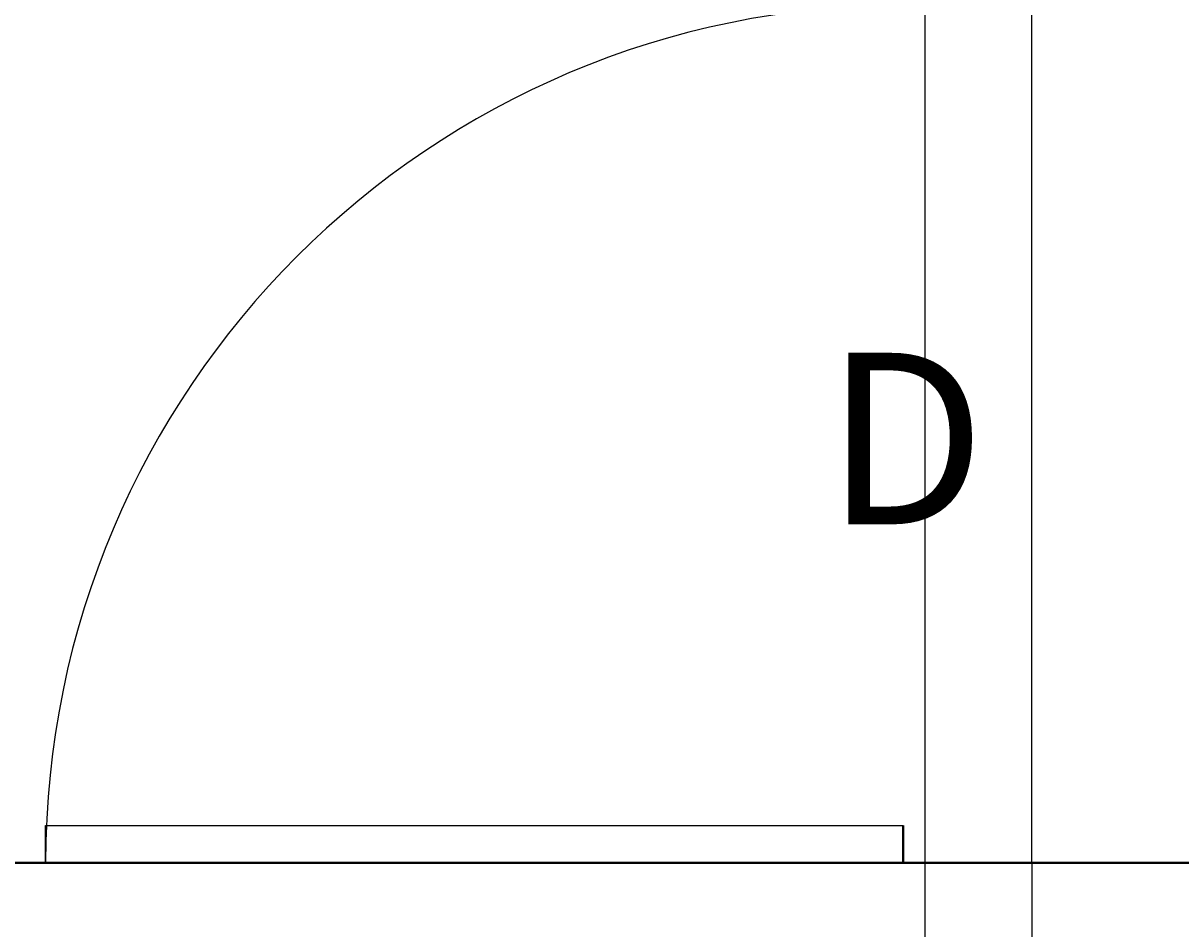
# Model space of a CAD drawing. Units: inches. Extents: x -301 to 715, y -607 to 364.
# Tile 65 of 141: x -93 to -39, y -218 to -176. Entities that reach past the tile are written whole.
import ezdxf

# ---------------------------------------------------------------- set-up
doc = ezdxf.new("R2010")
doc.units = ezdxf.units.IN
doc.header["$MEASUREMENT"] = 0
for name, color, linetype, lineweight in [('A-ANNO-DIMS', 2, 'Continuous', 18), ('A-ANNO-TEXT', 4, 'Continuous', 18), ('A-DOOR', 4, 'Continuous', 25), ('A-FLOR-STRS', 2, 'Continuous', 25), ('A-WALL', 3, 'Continuous', 40)]:
    doc.layers.add(name, color=color, linetype=linetype, lineweight=lineweight)
doc.styles.get("Standard").update_dxf_attribs({"font": 'arial.ttf'})
doc.dimstyles.get("Standard").update_dxf_attribs({"dimtxt": 0.18, "dimasz": 0.18, "dimexe": 0.18, "dimexo": 0.0625, "dimgap": 0.09, "dimtad": 0, "dimtih": 1, "dimtoh": 1, "dimdec": 1, "dimzin": 0, "dimdsep": 46, "dimlunit": 4, "dimtxsty": 'Standard', "dimcen": 0.09, "dimclrd": 3, "dimclre": 4, "dimclrt": 6, "dimadec": 0, "dimazin": 0, "dimtfac": 1, "dimtdec": 1, "dimtofl": 0, "dimtmove": 0, "dimatfit": 3, "dimfxl": 1, "dimtfill": 2, "dimtfillclr": 51, "dimtolj": 1, "dimtzin": 0, "dimarcsym": 0})

# ---------------------------------------------------------------- blocks, each defined once
blk = doc.blocks.new('*U4')
for p, q in [((0, 0), (0, -6)), ((40, 0), (40, -6))]:
    blk.add_line(p, q)
blk.add_lwpolyline([(0, 0), (0, 40), (1.75, 40), (1.75, 0)], close=True)
blk.add_arc((0, 0), 40, 0, 90)
blk = doc.blocks.new('ENTRY-STEPS-48')
for p, q in [((0, 27), (0, 18)), ((48, 27), (48, 18)), ((0, 18), (0, 9)), ((48, 9), (48, 18)), ((0, 9), (48, 9)), ((0, 9), (0, 0)), ((48, 0), (48, 9)), ((0, 0), (48, 0))]:
    blk.add_line(p, q)
blk = doc.blocks.new('*D151')
at = {"layer": 'A-ANNO-DIMS', "color": 4, "lineweight": -2, "transparency": 16777216}
for p, q in [((-204.603, -223.755), (-204.603, 359.612)), ((-45.603, -214.755), (-45.603, 359.612))]:
    blk.add_line(p, q, dxfattribs=at)
at = {"layer": 'A-ANNO-DIMS', "color": 3, "lineweight": -2, "transparency": 16777216}
for p, q in [((-204.423, 359.432), (-125.494, 359.432)), ((-45.783, 359.432), (-124.713, 359.432))]:
    blk.add_line(p, q, dxfattribs=at)
at = {"layer": 'A-ANNO-DIMS', "color": 3, "transparency": 16777216}
for points in [[(-204.423, 359.462), (-204.423, 359.402), (-204.603, 359.432)], [(-45.783, 359.462), (-45.783, 359.402), (-45.603, 359.432)]]:
    blk.add_solid(points, dxfattribs=at)
at = {"layer": 'Defpoints', "color": 0, "transparency": 16777216}
for p in [(-45.603, 359.432), (-45.603, -214.818), (-204.603, -223.818)]:
    blk.add_point(p, dxfattribs=at)
at = {"layer": 'A-ANNO-DIMS', "color": 6, "transparency": 16777216, "insert": (-125.103, 359.432), "char_height": 0.18, "attachment_point": 5, "bg_fill": 1, "box_fill_scale": 1.25, "bg_fill_color": 51, "bg_fill_transparency": 0}
blk.add_mtext('\\A1;13\'-3"', dxfattribs=at)
blk = doc.blocks.new('*D158')
at = {"layer": 'A-ANNO-DIMS', "color": 4, "lineweight": -2, "transparency": 16777216}
for p, q in [((-122.603, 221.62), (-122.603, -296.865)), ((-50.603, 221.62), (-50.603, -296.865))]:
    blk.add_line(p, q, dxfattribs=at)
at = {"layer": 'A-ANNO-DIMS', "color": 3, "lineweight": -2, "transparency": 16777216}
for p, q in [((-122.423, -296.685), (-86.933, -296.685)), ((-50.783, -296.685), (-86.274, -296.685))]:
    blk.add_line(p, q, dxfattribs=at)
at = {"layer": 'A-ANNO-DIMS', "color": 3, "transparency": 16777216}
for points in [[(-122.423, -296.655), (-122.423, -296.715), (-122.603, -296.685)], [(-50.783, -296.655), (-50.783, -296.715), (-50.603, -296.685)]]:
    blk.add_solid(points, dxfattribs=at)
at = {"layer": 'Defpoints', "color": 0, "transparency": 16777216}
for p in [(-122.603, 221.682), (-50.603, 221.682), (-50.603, -296.685)]:
    blk.add_point(p, dxfattribs=at)
at = {"layer": 'A-ANNO-DIMS', "color": 6, "transparency": 16777216, "insert": (-86.603, -296.685), "char_height": 0.18, "attachment_point": 5, "bg_fill": 1, "box_fill_scale": 1.25, "bg_fill_color": 51, "bg_fill_transparency": 0}
blk.add_mtext('\\A1;6\'-0"', dxfattribs=at)

msp = doc.modelspace()

# ---------------------------------------------------------------- linework, layer by layer
at = {"layer": 'A-WALL'}
for p, q in [((-51.603, -214.818), (-51.603, -213.068)), ((-195.603, -214.818), (-45.603, -214.818)), ((-45.841, -214.818), (123.897, -214.818))]:
    msp.add_line(p, q, dxfattribs=at)

# ---------------------------------------------------------------- block references
at = {"layer": 'A-DOOR', "rotation": 90}
msp.add_blockref('*U4', (-51.603, -214.818), dxfattribs=at)
at = {"layer": 'A-FLOR-STRS'}
msp.add_blockref('ENTRY-STEPS-48', (-45.603, -241.818), dxfattribs=at)

# ---------------------------------------------------------------- texts
at = {"layer": 'A-ANNO-TEXT'}
msp.add_text('D', height=8, dxfattribs=at).set_placement((-55.264, -199.026))

# ---------------------------------------------------------------- dimensions: what is measured, and where the dimension line sits
at = {"layer": 'A-ANNO-DIMS'}
for base, p1, p2, picture, middle in [((-45.603, 359.432), (-204.603, -223.818), (-45.603, -214.818), '*D151', (-125.103, 359.432)), ((-50.603, -296.685), (-122.603, 221.682), (-50.603, 221.682), '*D158', (-86.603, -296.685))]:
    dim = msp.add_linear_dim(base=base, p1=p1, p2=p2, dimstyle='Standard', override={"dimdec": 1, "dimlfac": 1, "dimrnd": 0, "dimzin": 1, "dimdsep": 46, "dimlunit": 4, "dimfrac": 2}, dxfattribs=at)
    dim.commit()
    dim.dimension.update_dxf_attribs({"geometry": picture, "text_midpoint": middle})

doc.saveas('drawing.dxf')
